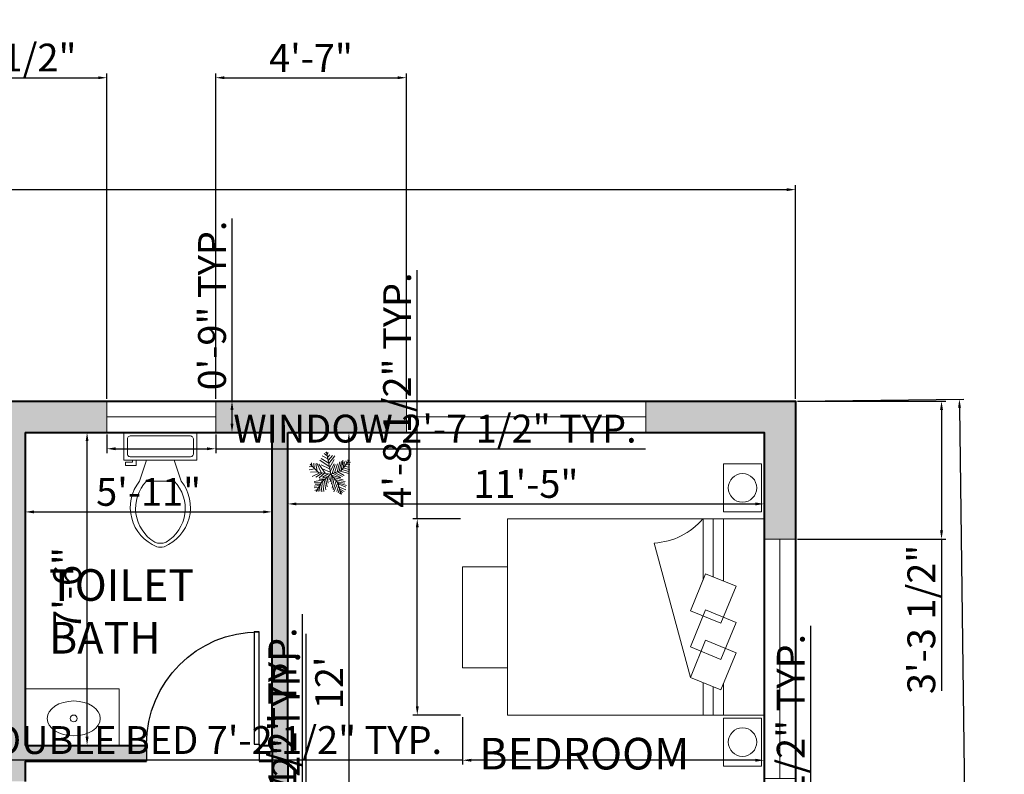
# Model space of a CAD drawing. Units: inches. Extents: x 529 to 1442, y 1029 to 1677.
# Tile 7 of 7: x 1135 to 1418, y 1460 to 1677. Entities that reach past the tile are written whole.
import ezdxf

# ---------------------------------------------------------------- set-up
doc = ezdxf.new("R2010")
doc.units = ezdxf.units.IN
for name, color, linetype, lineweight in [('A-ANNO-DIMS', 2, 'Continuous', 18), ('A-AREA-IDEN', 7, 'Continuous', 25), ('A-DOOR', 4, 'Continuous', 25), ('A-FLOR-FIXT', 9, 'Continuous', 18), ('A-FURN', 8, 'Continuous', 18), ('A-WALL-PATT', 252, 'Continuous', 13), ('tree', 70, 'Continuous', 13), ('wall', 7, 'Continuous', 40), ('window', 52, 'Continuous', 18)]:
    doc.layers.add(name, color=color, linetype=linetype, lineweight=lineweight)
doc.styles.get("Standard").update_dxf_attribs({"font": 'arial.ttf'})
doc.dimstyles.new('ISO-25', dxfattribs={"dimtxt": 8, "dimasz": 2.5, "dimexe": 1.25, "dimexo": 0.625, "dimtad": 1, "dimdec": 0, "dimlunit": 4, "dimtxsty": 'Standard', "dimcen": 2.5, "dimadec": 0, "dimazin": 0, "dimtfac": 1, "dimtdec": 0, "dimtmove": 0, "dimatfit": 3, "dimfxl": 1, "dimarcsym": 0})

# ---------------------------------------------------------------- blocks, each defined once
blk = doc.blocks.new('*U2')
for p, q in [((0, 0), (0, -6)), ((40, 0), (40, -6))]:
    blk.add_line(p, q)
blk.add_lwpolyline([(0, 0), (0, 40), (1.75, 40), (1.75, 0)], close=True)
blk.add_arc((0, 0), 40, 0, 90)
blk = doc.blocks.new('*U4')
for p, q in [((9.5, -6), (9.5, -2)), ((-8, -8.5), (-8, -8)), ((-7, -8), (-7, -9.5)), ((-4, -8), (-6, -14)), ((4, -8), (6, -14)), ((-10, -8.5), (-8, -8.5)), ((-10, -9.5), (-10, -8.5)), ((-7, -9.5), (-10, -9.5)), ((4, -14), (-4, -14))]:
    blk.add_line(p, q)
blk.add_lwpolyline([(10.5, -8), (10.5, 0), (-10.5, 0), (-10.5, -8)], close=True)
for points in [[(-9.5, -2), (-9.5, -6)], [(8.5, -1), (-8.5, -1)], [(-8.5, -7), (8.5, -7)]]:
    blk.add_lwpolyline(points)
for centre, radius, start, end in [((-8.62, -1.88), 0.884, 81.8699, 188.1301), ((8.62, -1.88), 0.884, 351.8699, 98.1301), ((-8.62, -6.12), 0.884, 171.8699, 278.1301), ((8.62, -6.12), 0.884, 261.8699, 8.1301), ((3.52, -21.58), 12.17, 141.4691, 247.9714), ((4.2, -21.82), 11.33, 136.3677, 238.9468), ((-3.52, -21.58), 12.17, 292.0284, 38.5307), ((-4.2, -21.82), 11.33, 301.053, 43.6321), ((0, -27.88), 4, 245.7318, 294.2682), ((0, -29), 4, 254.8605, 285.1395)]:
    blk.add_arc(centre, radius, start, end)
blk = doc.blocks.new('*U12')
for p, q in [((-8.737, 47.138), (-17.069, 52.711)), ((-10.186, 53.64), (-13.084, 55.962)), ((0, 0), (-10.5, 57)), ((-9.099, 51.782), (-6.563, 55.962)), ((-31.5, 4.5), (-52.5, 25.5)), ((-48.585, 21.131), (-49.309, 29.026)), ((-43.513, 28.561), (-42.427, 15.558)), ((-38.442, 26.239), (-34.819, 7.663)), ((-35.544, 28.097), (-24.314, 3.947)), ((-3.665, 19.273), (-27.574, 35.527)), ((-5.114, 28.097), (-24.676, 40.636)), ((-7.288, 39.707), (-21.778, 46.673)), ((-7.65, 43.423), (-2.578, 49.46)), ((-5.839, 35.992), (4.667, 48.067)), ((-5.114, 27.632), (10.463, 46.673)), ((-2.941, 16.486), (8.652, 37.85)), ((-1.129, 6.734), (9.014, 26.704)), ((10.101, 3.483), (17.708, 26.239)), ((16.259, 5.805), (23.142, 31.348)), ((22.055, 7.198), (27.489, 32.277)), ((27, 9), (48, 36)), ((27.127, 9.056), (31.112, 35.992)), ((31.836, 30.883), (32.561, 16.486)), ((35.096, 32.741), (37.27, 22.524)), ((38.719, 34.134), (41.979, 28.561)), ((40.53, 25.775), (48.862, 24.846)), ((43.791, 29.954), (51.036, 30.883)), ((44.153, 36.456), (45.239, 32.741)), ((-47.498, 19.737), (-55.83, 18.344)), ((-40.615, 13.7), (-55.105, 10.913)), ((-33.37, 6.269), (-52.207, 5.34)), ((-28.299, 3.483), (-47.86, -5.805)), ((-21.416, 3.018), (-38.079, -8.128)), ((0, 0), (-31.5, 4.5)), ((-14.533, 2.09), (-30.834, 25.31)), ((-15.982, 2.09), (-30.11, -9.521)), ((-24.314, 23.917), (-2.941, 13.7)), ((0, 0), (-22.5, -19.5)), ((-6.563, 1.161), (-21.416, -8.128)), ((-20.691, 13.7), (-1.129, 4.876)), ((0, 0), (27, 9)), ((0, 0), (18, -22.5)), ((3.942, 1.625), (11.187, 24.381)), ((6.478, 1.625), (26.04, -8.592)), ((11.187, 3.483), (30.749, -5.805)), ((18.07, 5.805), (35.096, -3.483)), ((24.229, 7.663), (46.688, 1.625)), ((29.662, 12.307), (48.137, 6.269)), ((33.285, 16.486), (48.862, 10.913)), ((36.183, 19.737), (48.137, 17.88)), ((-17.431, -15.094), (-42.789, -18.809)), ((-24.314, -21.596), (-42.427, -22.06)), ((-22.5, -19.5), (-37.5, -45)), ((-15.257, -12.772), (-30.11, -12.772)), ((-25.038, -23.918), (-22.865, -45.281)), ((-20.691, -18.345), (-17.793, -44.352)), ((-6.563, -5.805), (-19.967, -9.985)), ((-17.069, -15.094), (-12.721, -40.172)), ((-13.446, -11.378), (-8.737, -32.741)), ((-9.461, -8.592), (-6.201, -23.453)), ((-4.752, -3.483), (-3.665, -14.629)), ((2.493, -3.019), (-1.491, -20.202)), ((1.769, -2.555), (24.229, -9.521)), ((5.029, -6.27), (2.131, -25.775)), ((9.014, -11.378), (3.58, -35.992)), ((14.085, -16.951), (6.478, -40.172)), ((7.565, -9.056), (32.198, -14.629)), ((18.07, -22.524), (8.289, -45.745)), ((12.274, -15.094), (36.907, -18.809)), ((16.259, -19.738), (36.183, -22.989)), ((18, -22.5), (27, -52.5)), ((18.433, -22.524), (40.53, -29.026)), ((19.157, -25.311), (38.719, -33.206)), ((-28.299, -29.026), (-42.789, -31.348)), ((-30.834, -34.135), (-42.427, -35.528)), ((-34.457, -39.708), (-40.978, -42.494)), ((-26.849, -26.24), (-40.253, -25.775)), ((-32.646, -36.921), (-31.921, -44.352)), ((-29.023, -30.884), (-27.936, -43.887)), ((20.244, -30.419), (15.897, -44.816)), ((22.78, -37.85), (19.519, -48.532)), ((21.331, -32.741), (39.081, -40.636)), ((22.78, -38.314), (34.372, -44.816)), ((24.591, -45.745), (23.142, -50.854)), ((24.591, -43.423), (30.749, -47.603)), ((26.764, -49.925), (28.213, -50.854))]:
    blk.add_line(p, q)
blk = doc.blocks.new('*D21')
at = {"layer": 'A-ANNO-DIMS', "color": 0, "lineweight": -2, "transparency": 16777216}
for p, q in [((1136.88, 1557.19), (1136.88, 1533.72)), ((1207.88, 1557.19), (1207.88, 1533.72)), ((1139.38, 1534.97), (1205.38, 1534.97))]:
    blk.add_line(p, q, dxfattribs=at)
at = {"layer": 'A-ANNO-DIMS', "color": 0, "lineweight": 100, "transparency": 16777216}
for points in [[(1139.38, 1535.38), (1139.38, 1534.55), (1136.88, 1534.97)], [(1205.38, 1535.38), (1205.38, 1534.55), (1207.88, 1534.97)]]:
    blk.add_solid(points, dxfattribs=at)
at = {"layer": 'Defpoints', "color": 0, "lineweight": 100, "transparency": 16777216}
for p in [(1136.88, 1557.81), (1207.88, 1557.81), (1207.88, 1534.97)]:
    blk.add_point(p, dxfattribs=at)
at = {"layer": 'A-ANNO-DIMS', "color": 0, "transparency": 16777216, "insert": (1172.38, 1539.68), "char_height": 8, "attachment_point": 5}
blk.add_mtext('5\'-11"', dxfattribs=at)
blk = doc.blocks.new('*D22')
at = {"layer": 'A-ANNO-DIMS', "color": 0, "lineweight": -2, "transparency": 16777216}
for p, q in [((1137.51, 1557.81), (1155.94, 1557.81)), ((1154.69, 1470.31), (1154.69, 1555.31)), ((1137.51, 1467.81), (1155.94, 1467.81))]:
    blk.add_line(p, q, dxfattribs=at)
at = {"layer": 'A-ANNO-DIMS', "color": 0, "lineweight": 100, "transparency": 16777216}
for points in [[(1154.27, 1555.31), (1155.1, 1555.31), (1154.69, 1557.81)], [(1154.27, 1470.31), (1155.1, 1470.31), (1154.69, 1467.81)]]:
    blk.add_solid(points, dxfattribs=at)
at = {"layer": 'Defpoints', "color": 0, "lineweight": 100, "transparency": 16777216}
for p in [(1136.88, 1557.81), (1154.69, 1557.81), (1136.88, 1467.81)]:
    blk.add_point(p, dxfattribs=at)
at = {"layer": 'A-ANNO-DIMS', "color": 0, "transparency": 16777216, "insert": (1149.98, 1512.81), "char_height": 8, "attachment_point": 5, "rotation": 90}
blk.add_mtext('7\'-6"', dxfattribs=at)
blk = doc.blocks.new('*D23')
at = {"layer": 'A-ANNO-DIMS', "color": 0, "lineweight": -2, "transparency": 16777216}
for p, q in [((1212.38, 1557.19), (1212.38, 1536.01)), ((1349.38, 1557.19), (1349.38, 1536.01)), ((1214.88, 1537.26), (1346.88, 1537.26))]:
    blk.add_line(p, q, dxfattribs=at)
at = {"layer": 'A-ANNO-DIMS', "color": 0, "lineweight": 100, "transparency": 16777216}
for points in [[(1214.88, 1537.68), (1214.88, 1536.85), (1212.38, 1537.26)], [(1346.88, 1537.68), (1346.88, 1536.85), (1349.38, 1537.26)]]:
    blk.add_solid(points, dxfattribs=at)
at = {"layer": 'Defpoints', "color": 0, "lineweight": 100, "transparency": 16777216}
for p in [(1212.38, 1557.81), (1349.38, 1557.81), (1349.38, 1537.26)]:
    blk.add_point(p, dxfattribs=at)
at = {"layer": 'A-ANNO-DIMS', "color": 0, "transparency": 16777216, "insert": (1280.88, 1541.97), "char_height": 8, "attachment_point": 5}
blk.add_mtext('11\'-5"', dxfattribs=at)
blk = doc.blocks.new('*D24')
at = {"layer": 'A-ANNO-DIMS', "color": 0, "lineweight": -2, "transparency": 16777216}
for p, q in [((1348.76, 1557.81), (1228.73, 1557.81)), ((1229.98, 1555.31), (1229.98, 1416.31)), ((1348.76, 1413.81), (1228.73, 1413.81))]:
    blk.add_line(p, q, dxfattribs=at)
at = {"layer": 'A-ANNO-DIMS', "color": 0, "lineweight": 100, "transparency": 16777216}
for points in [[(1229.56, 1555.31), (1230.39, 1555.31), (1229.98, 1557.81)], [(1229.56, 1416.31), (1230.39, 1416.31), (1229.98, 1413.81)]]:
    blk.add_solid(points, dxfattribs=at)
at = {"layer": 'Defpoints', "color": 0, "lineweight": 100, "transparency": 16777216}
for p in [(1349.38, 1557.81), (1229.98, 1413.81), (1349.38, 1413.81)]:
    blk.add_point(p, dxfattribs=at)
at = {"layer": 'A-ANNO-DIMS', "color": 0, "transparency": 16777216, "insert": (1225.34, 1485.81), "char_height": 8, "attachment_point": 5, "rotation": 90}
blk.add_mtext("12'", dxfattribs=at)
blk = doc.blocks.new('*D55')
at = {"layer": 'A-ANNO-DIMS', "color": 0, "lineweight": -2, "transparency": 16777216}
for p, q in [((638.38, 1567.44), (638.38, 1628.88)), ((1358.38, 1567.44), (1358.38, 1628.88)), ((640.88, 1627.63), (1355.88, 1627.63))]:
    blk.add_line(p, q, dxfattribs=at)
at = {"layer": 'A-ANNO-DIMS', "color": 0, "lineweight": 100, "transparency": 16777216}
for points in [[(640.88, 1628.05), (640.88, 1627.22), (638.38, 1627.63)], [(1355.88, 1628.05), (1355.88, 1627.22), (1358.38, 1627.63)]]:
    blk.add_solid(points, dxfattribs=at)
at = {"layer": 'Defpoints', "color": 0, "lineweight": 100, "transparency": 16777216}
for p in [(1358.38, 1627.63), (638.38, 1566.81), (1358.38, 1566.81)]:
    blk.add_point(p, dxfattribs=at)
at = {"layer": 'A-ANNO-DIMS', "color": 0, "transparency": 16777216, "insert": (998.38, 1632.34), "char_height": 8, "attachment_point": 5}
blk.add_mtext("60'", dxfattribs=at)
blk = doc.blocks.new('*D56')
at = {"layer": 'A-ANNO-DIMS', "color": 0, "lineweight": -2, "transparency": 16777216}
for p, q in [((1359.01, 1566.82), (1406.77, 1567.43)), ((1405.56, 1564.91), (1410.83, 1149.91)), ((1364.34, 1146.82), (1412.11, 1147.43))]:
    blk.add_line(p, q, dxfattribs=at)
at = {"layer": 'A-ANNO-DIMS', "color": 0, "lineweight": 100, "transparency": 16777216}
for points in [[(1405.97, 1564.92), (1405.14, 1564.91), (1405.52, 1567.41)], [(1411.24, 1149.92), (1410.41, 1149.91), (1410.86, 1147.41)]]:
    blk.add_solid(points, dxfattribs=at)
at = {"layer": 'Defpoints', "color": 0, "lineweight": 100, "transparency": 16777216}
for p in [(1358.38, 1566.81), (1363.72, 1146.81), (1410.86, 1147.41)]:
    blk.add_point(p, dxfattribs=at)
at = {"layer": 'A-ANNO-DIMS', "color": 0, "transparency": 16777216, "insert": (1412.9, 1357.47), "char_height": 8, "attachment_point": 5, "rotation": 270.7276}
blk.add_mtext("35'", dxfattribs=at)
blk = doc.blocks.new('WIN-LARGE-PLAN')
blk.add_line((0, 4.5), (68.85, 4.5))
blk.add_lwpolyline([(0, 9), (68.85, 9), (68.85, 0), (0, 0)], close=True)
blk = doc.blocks.new('WIN-SMALL-PLAN')
blk.add_line((0, 4.5), (31.29, 4.5))
blk.add_lwpolyline([(0, 9), (31.29, 9), (31.29, 0), (0, 0)], close=True)
blk = doc.blocks.new('BED-DOUBLE')
for p, q in [((10.82, 21.21), (49.46, 31.61)), ((0, 17.58), (9.33, 17.58)), ((0, 17.58), (9.33, 17.58)), ((28.37, 17.58), (28.47, 17.58)), ((28.37, 17.58), (28.47, 17.58)), ((38.76, 17.58), (56.44, 17.58)), ((38.76, 17.58), (56.44, 17.58)), ((0, 14.65), (8.12, 14.65)), ((39.74, 14.65), (56.44, 14.65)), ((0, 11.71), (9.09, 11.71)), ((28.13, 11.71), (28.23, 11.71)), ((38.53, 11.71), (56.44, 11.71))]:
    blk.add_line(p, q)
for points in [[(13.54, 73.79), (42.58, 73.79), (42.58, 86.74), (13.54, 86.74)], [(0, 0), (56.44, 0), (56.44, 73.79), (0, 73.79)], [(10.82, 21.21), (21.49, 16.82), (17.9, 8.09), (7.23, 12.48)], [(19.56, 21.21), (30.23, 16.82), (26.64, 8.09), (15.97, 12.48)], [(29.96, 21.21), (40.63, 16.82), (37.04, 8.09), (26.37, 12.48)]]:
    blk.add_lwpolyline(points, close=True)
blk.add_arc((69.23, 32.7), 19.8, 183.1428, 229.758)
blk = doc.blocks.new('NIGHTSTAND')
blk.add_lwpolyline([(0, 0), (13.77, 0), (13.77, 10.99), (0, 10.99)], close=True)
blk.add_circle((6.88, 5.5), 4.1)
blk = doc.blocks.new('WASHBASIN')
blk.add_lwpolyline([(0, 16.29), (27.02, 16.29), (27.02, 0), (0, 0)], close=True)
blk.add_circle((13.05, 8.54), 0.991)
blk.add_ellipse((13.05, 8.54), major_axis=(7.63, 0), ratio=0.659433)
blk = doc.blocks.new('*D73')
at = {"layer": 'A-ANNO-DIMS', "color": 0, "lineweight": -2, "transparency": 16777216}
for p, q in [((1160.38, 1557.19), (1160.38, 1551.87)), ((1191.67, 1557.19), (1191.67, 1551.87)), ((1162.88, 1553.12), (1189.17, 1553.12)), ((1191.67, 1553.12), (1315.29, 1553.12))]:
    blk.add_line(p, q, dxfattribs=at)
at = {"layer": 'A-ANNO-DIMS', "color": 0, "lineweight": 100, "transparency": 16777216}
for points in [[(1162.88, 1553.54), (1162.88, 1552.7), (1160.38, 1553.12)], [(1189.17, 1553.54), (1189.17, 1552.7), (1191.67, 1553.12)]]:
    blk.add_solid(points, dxfattribs=at)
at = {"layer": 'Defpoints', "color": 0, "lineweight": 100, "transparency": 16777216}
for p in [(1160.38, 1557.81), (1191.67, 1557.81), (1191.67, 1553.12)]:
    blk.add_point(p, dxfattribs=at)
at = {"layer": 'A-ANNO-DIMS', "color": 0, "transparency": 16777216, "insert": (1254.73, 1557.88), "char_height": 8, "attachment_point": 5}
blk.add_mtext('WINDOW 2\'-7 1/2" TYP.', dxfattribs=at)
blk = doc.blocks.new('*D74')
at = {"layer": 'A-ANNO-DIMS', "color": 0, "lineweight": -2, "transparency": 16777216}
for p, q in [((1196.36, 1566.81), (1196.36, 1619.33)), ((1192.29, 1566.81), (1197.61, 1566.81)), ((1196.36, 1560.31), (1196.36, 1564.31)), ((1192.29, 1557.81), (1197.61, 1557.81))]:
    blk.add_line(p, q, dxfattribs=at)
at = {"layer": 'A-ANNO-DIMS', "color": 0, "lineweight": 100, "transparency": 16777216}
for points in [[(1195.94, 1564.31), (1196.78, 1564.31), (1196.36, 1566.81)], [(1195.94, 1560.31), (1196.78, 1560.31), (1196.36, 1557.81)]]:
    blk.add_solid(points, dxfattribs=at)
at = {"layer": 'Defpoints', "color": 0, "lineweight": 100, "transparency": 16777216}
for p in [(1191.67, 1566.81), (1196.36, 1566.81), (1191.67, 1557.81)]:
    blk.add_point(p, dxfattribs=at)
at = {"layer": 'A-ANNO-DIMS', "color": 0, "transparency": 16777216, "insert": (1191.65, 1594.32), "char_height": 8, "attachment_point": 5, "rotation": 90}
blk.add_mtext('0\'-9" TYP.', dxfattribs=at)
blk = doc.blocks.new('*D75')
at = {"layer": 'A-ANNO-DIMS', "color": 0, "lineweight": -2, "transparency": 16777216}
for p, q in [((1362.81, 1397.77), (1362.81, 1502.25)), ((1359.01, 1397.77), (1364.06, 1397.77)), ((1362.81, 1370.77), (1362.81, 1395.27)), ((1359.01, 1368.27), (1364.06, 1368.27))]:
    blk.add_line(p, q, dxfattribs=at)
at = {"layer": 'A-ANNO-DIMS', "color": 0, "lineweight": 100, "transparency": 16777216}
for points in [[(1362.39, 1395.27), (1363.23, 1395.27), (1362.81, 1397.77)], [(1362.39, 1370.77), (1363.23, 1370.77), (1362.81, 1368.27)]]:
    blk.add_solid(points, dxfattribs=at)
at = {"layer": 'Defpoints', "color": 0, "lineweight": 100, "transparency": 16777216}
for p in [(1358.38, 1397.77), (1362.81, 1397.77), (1358.38, 1368.27)]:
    blk.add_point(p, dxfattribs=at)
at = {"layer": 'A-ANNO-DIMS', "color": 0, "transparency": 16777216, "insert": (1358.05, 1451.26), "char_height": 8, "attachment_point": 5, "rotation": 90}
blk.add_mtext('VENT 2\'-5 1/2" TYP.', dxfattribs=at)
blk = doc.blocks.new('*D77')
at = {"layer": 'A-ANNO-DIMS', "color": 0, "lineweight": -2, "transparency": 16777216}
for p, q in [((1262.64, 1475.94), (1262.64, 1462.3)), ((1349.38, 1475.94), (1349.38, 1462.3)), ((1262.64, 1463.55), (1116.74, 1463.55)), ((1346.88, 1463.55), (1265.14, 1463.55))]:
    blk.add_line(p, q, dxfattribs=at)
at = {"layer": 'A-ANNO-DIMS', "color": 0, "lineweight": 100, "transparency": 16777216}
for points in [[(1265.14, 1463.97), (1265.14, 1463.13), (1262.64, 1463.55)], [(1346.88, 1463.97), (1346.88, 1463.13), (1349.38, 1463.55)]]:
    blk.add_solid(points, dxfattribs=at)
at = {"layer": 'Defpoints', "color": 0, "lineweight": 100, "transparency": 16777216}
for p in [(1262.64, 1476.56), (1349.38, 1476.56), (1262.64, 1463.55)]:
    blk.add_point(p, dxfattribs=at)
at = {"layer": 'A-ANNO-DIMS', "color": 0, "transparency": 16777216, "insert": (1188.44, 1468.32), "char_height": 8, "attachment_point": 5}
blk.add_mtext('DOUBLE BED 7\'-2 1/2" TYP.', dxfattribs=at)
blk = doc.blocks.new('*D78')
at = {"layer": 'A-ANNO-DIMS', "color": 0, "lineweight": -2, "transparency": 16777216}
for p, q in [((1249.63, 1533), (1249.63, 1604.48)), ((1262.02, 1533), (1248.38, 1533)), ((1249.63, 1479.06), (1249.63, 1530.5)), ((1262.02, 1476.56), (1248.38, 1476.56))]:
    blk.add_line(p, q, dxfattribs=at)
at = {"layer": 'A-ANNO-DIMS', "color": 0, "lineweight": 100, "transparency": 16777216}
for points in [[(1249.22, 1530.5), (1250.05, 1530.5), (1249.63, 1533)], [(1249.22, 1479.06), (1250.05, 1479.06), (1249.63, 1476.56)]]:
    blk.add_solid(points, dxfattribs=at)
at = {"layer": 'Defpoints', "color": 0, "lineweight": 100, "transparency": 16777216}
for p in [(1249.63, 1533), (1262.64, 1533), (1262.64, 1476.56)]:
    blk.add_point(p, dxfattribs=at)
at = {"layer": 'A-ANNO-DIMS', "color": 0, "transparency": 16777216, "insert": (1244.87, 1569.99), "char_height": 8, "attachment_point": 5, "rotation": 90}
blk.add_mtext('4\'-8 1/2" TYP.', dxfattribs=at)
blk = doc.blocks.new('*D87')
at = {"layer": 'A-ANNO-DIMS', "color": 0, "lineweight": -2, "transparency": 16777216}
for p, q in [((1216.62, 1371.24), (1216.62, 1505.58)), ((1213.45, 1371.24), (1217.87, 1371.24)), ((1216.62, 1348.45), (1216.62, 1368.74)), ((1213.45, 1345.95), (1217.87, 1345.95))]:
    blk.add_line(p, q, dxfattribs=at)
at = {"layer": 'A-ANNO-DIMS', "color": 0, "lineweight": 100, "transparency": 16777216}
for points in [[(1216.2, 1368.74), (1217.04, 1368.74), (1216.62, 1371.24)], [(1216.2, 1348.45), (1217.04, 1348.45), (1216.62, 1345.95)]]:
    blk.add_solid(points, dxfattribs=at)
at = {"layer": 'Defpoints', "color": 0, "lineweight": 100, "transparency": 16777216}
for p in [(1212.83, 1371.24), (1216.62, 1371.24), (1212.83, 1345.95)]:
    blk.add_point(p, dxfattribs=at)
at = {"layer": 'A-ANNO-DIMS', "color": 0, "transparency": 16777216, "insert": (1211.86, 1439.66), "char_height": 8, "attachment_point": 5, "rotation": 90}
blk.add_mtext('ARMCHAIR 2\'-1 1/2" TYP.', dxfattribs=at)
blk = doc.blocks.new('*D91')
at = {"layer": 'A-ANNO-DIMS', "color": 0, "lineweight": -2, "transparency": 16777216}
for p, q in [((1217.67, 1335.7), (1217.67, 1499.91)), ((1212.96, 1335.7), (1218.92, 1335.7)), ((1217.67, 1302.63), (1217.67, 1333.2)), ((1212.96, 1300.13), (1218.92, 1300.13))]:
    blk.add_line(p, q, dxfattribs=at)
at = {"layer": 'A-ANNO-DIMS', "color": 0, "lineweight": 100, "transparency": 16777216}
for points in [[(1217.25, 1333.2), (1218.08, 1333.2), (1217.67, 1335.7)], [(1217.25, 1302.63), (1218.08, 1302.63), (1217.67, 1300.13)]]:
    blk.add_solid(points, dxfattribs=at)
at = {"layer": 'Defpoints', "color": 0, "lineweight": 100, "transparency": 16777216}
for p in [(1212.33, 1335.7), (1217.67, 1335.7), (1212.33, 1300.13)]:
    blk.add_point(p, dxfattribs=at)
at = {"layer": 'A-ANNO-DIMS', "color": 0, "transparency": 16777216, "insert": (1212.9, 1419.05), "char_height": 8, "attachment_point": 5, "rotation": 90}
blk.add_mtext('COFFEE TABLE 2\'-11 1/2" TYP.', dxfattribs=at)
blk = doc.blocks.new('*D103')
at = {"layer": 'A-ANNO-DIMS', "color": 0, "lineweight": -2, "transparency": 16777216}
for p, q in [((1099.95, 1567.44), (1099.95, 1661.06)), ((1102.45, 1659.81), (1157.88, 1659.81)), ((1160.38, 1567.44), (1160.38, 1661.06))]:
    blk.add_line(p, q, dxfattribs=at)
at = {"layer": 'A-ANNO-DIMS', "color": 0, "lineweight": 100, "transparency": 16777216}
for points in [[(1102.45, 1660.23), (1102.45, 1659.4), (1099.95, 1659.81)], [(1157.88, 1660.23), (1157.88, 1659.4), (1160.38, 1659.81)]]:
    blk.add_solid(points, dxfattribs=at)
at = {"layer": 'Defpoints', "color": 0, "lineweight": 100, "transparency": 16777216}
for p in [(1160.38, 1659.81), (1099.95, 1566.81), (1160.38, 1566.81)]:
    blk.add_point(p, dxfattribs=at)
at = {"layer": 'A-ANNO-DIMS', "color": 0, "transparency": 16777216, "insert": (1130.17, 1664.57), "char_height": 8, "attachment_point": 5}
blk.add_mtext('5\'-0 1/2"', dxfattribs=at)
blk = doc.blocks.new('*D104')
at = {"layer": 'A-ANNO-DIMS', "color": 0, "lineweight": -2, "transparency": 16777216}
for p, q in [((1191.67, 1567.44), (1191.67, 1661.06)), ((1194.17, 1659.81), (1244, 1659.81)), ((1246.5, 1567.44), (1246.5, 1661.06))]:
    blk.add_line(p, q, dxfattribs=at)
at = {"layer": 'A-ANNO-DIMS', "color": 0, "lineweight": 100, "transparency": 16777216}
for points in [[(1194.17, 1660.23), (1194.17, 1659.4), (1191.67, 1659.81)], [(1244, 1660.23), (1244, 1659.4), (1246.5, 1659.81)]]:
    blk.add_solid(points, dxfattribs=at)
at = {"layer": 'Defpoints', "color": 0, "lineweight": 100, "transparency": 16777216}
for p in [(1246.5, 1659.81), (1191.67, 1566.81), (1246.5, 1566.81)]:
    blk.add_point(p, dxfattribs=at)
at = {"layer": 'A-ANNO-DIMS', "color": 0, "transparency": 16777216, "insert": (1219.08, 1664.44), "char_height": 8, "attachment_point": 5}
blk.add_mtext('4\'-7"', dxfattribs=at)
blk = doc.blocks.new('*D108')
at = {"layer": 'A-ANNO-DIMS', "color": 0, "lineweight": -2, "transparency": 16777216}
for p, q in [((1359.01, 1566.81), (1401.63, 1566.81)), ((1400.38, 1564.31), (1400.38, 1529.64)), ((1359.01, 1527.14), (1401.63, 1527.14)), ((1400.38, 1527.14), (1400.38, 1483.49))]:
    blk.add_line(p, q, dxfattribs=at)
at = {"layer": 'A-ANNO-DIMS', "color": 0, "lineweight": 100, "transparency": 16777216}
for points in [[(1399.97, 1564.31), (1400.8, 1564.31), (1400.38, 1566.81)], [(1399.97, 1529.64), (1400.8, 1529.64), (1400.38, 1527.14)]]:
    blk.add_solid(points, dxfattribs=at)
at = {"layer": 'Defpoints', "color": 0, "lineweight": 100, "transparency": 16777216}
for p in [(1358.38, 1566.81), (1358.38, 1527.14), (1400.38, 1527.14)]:
    blk.add_point(p, dxfattribs=at)
at = {"layer": 'A-ANNO-DIMS', "color": 0, "transparency": 16777216, "insert": (1395.62, 1504.06), "char_height": 8, "attachment_point": 5, "rotation": 90}
blk.add_mtext('3\'-3 1/2"', dxfattribs=at)

msp = doc.modelspace()

# ---------------------------------------------------------------- hatches: boundary and pattern name
at = {"layer": 'A-WALL-PATT'}
h = msp.add_hatch(color=256, dxfattribs=at)
h.dxf.hatch_style = 1
h.paths.add_polyline_path([(1132.38, 1328.31), (1041.38, 1328.31), (1041.38, 1323.81), (1132.38, 1323.81)])
h.paths.add_polyline_path([(1132.38, 1413.81), (1075.12, 1413.81), (1075.12, 1409.31), (1132.38, 1409.31)])
h.paths.add_polyline_path([(1246.5, 1566.81), (1191.67, 1566.81), (1191.67, 1557.81), (1246.5, 1557.81)])
h.paths.add_polyline_path([(1160.38, 1566.81), (1099.95, 1566.81), (1099.95, 1557.81), (1132.38, 1557.81), (1160.38, 1557.81)])
h = msp.add_hatch(color=256, dxfattribs=at)
h.dxf.hatch_style = 1
h.paths.add_polyline_path([(1160.38, 1566.81), (1099.95, 1566.81), (1099.95, 1557.81), (1132.38, 1557.81), (1160.38, 1557.81)])
h.paths.add_polyline_path([(1136.88, 1557.81), (1132.38, 1557.81), (1132.38, 1457.46), (1136.88, 1457.46)])
h.paths.add_polyline_path([(1171.8, 1467.81), (1136.88, 1467.81), (1136.88, 1463.31), (1171.8, 1463.31)])
h.paths.add_polyline_path([(1212.38, 1557.81), (1207.88, 1557.81), (1207.88, 1467.81), (1207.88, 1409.31), (1218.04, 1409.31), (1218.04, 1413.81), (1212.38, 1413.81), (1212.38, 1463.31)])
h.paths.add_polyline_path([(1136.88, 1409.31), (1132.38, 1409.31), (1132.38, 1146.81), (1136.88, 1146.81)])
h.paths.add_polyline_path([(1136.88, 1417.46), (1132.38, 1417.46), (1132.38, 1409.31), (1136.88, 1409.31)])
h.paths.add_polyline_path([(1132.38, 1413.81), (1075.12, 1413.81), (1075.12, 1409.31), (1132.38, 1409.31)])
h.paths.add_polyline_path([(1132.38, 1328.31), (1041.38, 1328.31), (1041.38, 1323.81), (1132.38, 1323.81)])
h = msp.add_hatch(color=256, dxfattribs=at)
h.dxf.hatch_style = 1
h.paths.add_polyline_path([(1358.38, 1566.81), (1315.35, 1566.81), (1315.35, 1557.81), (1349.38, 1557.81), (1349.38, 1527.14), (1358.38, 1527.14)])
h = msp.add_hatch(color=256, dxfattribs=at)
h.dxf.hatch_style = 1
h.paths.add_polyline_path([(1171.8, 1467.81), (1136.88, 1467.81), (1136.88, 1463.31), (1171.8, 1463.31)])
h.paths.add_polyline_path([(1136.88, 1557.81), (1132.38, 1557.81), (1132.38, 1457.46), (1136.88, 1457.46)])
h.paths.add_polyline_path([(1212.38, 1557.81), (1207.88, 1557.81), (1207.88, 1467.81), (1207.88, 1409.31), (1218.04, 1409.31), (1218.04, 1413.81), (1212.38, 1413.81), (1212.38, 1463.31)])

# ---------------------------------------------------------------- linework, layer by layer
at = {"layer": 'wall'}
for p, q in [((638.38, 1566.81), (1358.38, 1566.81)), ((1358.38, 1566.81), (1358.38, 1146.81)), ((1136.88, 1557.81), (1136.88, 1467.81)), ((1136.88, 1557.81), (1136.88, 1467.81)), ((1207.88, 1467.81), (1207.88, 1557.81)), ((1212.38, 1463.31), (1212.38, 1557.81)), ((1349.38, 1557.81), (1349.38, 1413.81)), ((1136.88, 1467.81), (1171.8, 1467.81)), ((1204.13, 1467.81), (1207.88, 1467.81)), ((1207.88, 1467.81), (1207.88, 1409.31)), ((1136.88, 1463.31), (1171.8, 1463.31)), ((1136.88, 1463.31), (1136.88, 1457.46)), ((1204.13, 1463.31), (1207.88, 1463.31)), ((1212.38, 1463.31), (1212.38, 1413.81))]:
    msp.add_line(p, q, dxfattribs=at)
for points in [[(859.38, 1146.81), (638.38, 1146.81), (638.38, 1566.81), (1358.38, 1566.81), (1358.38, 1146.81), (1132.38, 1146.81)], [(1136.88, 1557.81), (1207.88, 1557.81)], [(1212.38, 1557.81), (1349.38, 1557.81), (1349.38, 1253.97)]]:
    msp.add_lwpolyline(points, dxfattribs=at)

# ---------------------------------------------------------------- block references
at = {"layer": 'A-DOOR', "xscale": -0.8082241798979204, "yscale": 0.8082241798979204, "zscale": 0.8082241798979204}
msp.add_blockref('*U2', (1204.13, 1468.16), dxfattribs=at)
at = {"layer": 'A-FLOR-FIXT'}
msp.add_blockref('*U4', (1175.77, 1557.81), dxfattribs=at)
at = {"layer": 'A-FLOR-FIXT', "rotation": 180}
msp.add_blockref('WASHBASIN', (1163.9, 1484.1), dxfattribs=at)
msp.add_blockref('WASHBASIN', (1163.9, 1484.1), dxfattribs=at)
at = {"layer": 'A-FURN'}
for name, p, rotation in [('NIGHTSTAND', (1348.66, 1534.99), 89.99999999999616), ('BED-DOUBLE', (1349.38, 1476.56), 90.0000000000003), ('NIGHTSTAND', (1348.66, 1461.89), 89.99999999999456)]:
    msp.add_blockref(name, p, dxfattribs=dict(at, rotation=rotation))
at = {"layer": 'tree', "xscale": 0.1116431773080361, "yscale": 0.1116431773080361, "zscale": 0.1116431773080361}
msp.add_blockref('*U12', (1224.74, 1545.83), dxfattribs=at)
at = {"layer": 'window'}
for name, p in [('WIN-SMALL-PLAN', (1160.38, 1557.81)), ('WIN-LARGE-PLAN', (1246.5, 1557.81))]:
    msp.add_blockref(name, p, dxfattribs=at)
at = {"layer": 'window', "rotation": 269.9999999999987}
msp.add_blockref('WIN-LARGE-PLAN', (1349.38, 1527.14), dxfattribs=at)

# ---------------------------------------------------------------- texts
at = {"layer": 'A-AREA-IDEN', "char_height": 9.098, "attachment_point": 1}
for s, insert in [('TOILET\\PBATH', (1143.71, 1518.49)), ('BEDROOM', (1267.45, 1469.99))]:
    msp.add_mtext_dynamic_manual_height_columns(s, width=307.5887, gutter_width=45.49, heights=[0], dxfattribs=dict(at, insert=insert))

# ---------------------------------------------------------------- dimensions: what is measured, and where the dimension line sits
at = {"layer": 'A-ANNO-DIMS'}
for base, p1, p2, override, picture, middle in [((1160.38, 1659.81), (1099.95, 1566.81), (1160.38, 1566.81), {"dimdec": 1, "dimlfac": 1, "dimrnd": 0, "dimzin": 1, "dimdsep": 46, "dimlunit": 4, "dimfrac": 2}, '*D103', (1130.17, 1664.57)), ((1246.5, 1659.81), (1191.67, 1566.81), (1246.5, 1566.81), {"dimdec": 1, "dimlfac": 1, "dimrnd": 0, "dimzin": 1, "dimdsep": 46, "dimlunit": 4, "dimfrac": 2}, '*D104', (1219.08, 1664.44)), ((1358.38, 1627.63), (638.38, 1566.81), (1358.38, 1566.81), {"dimclrd": 0, "dimclre": 0, "dimclrt": 0}, '*D55', (998.38, 1632.34)), ((1207.88, 1534.97), (1136.88, 1557.81), (1207.88, 1557.81), {"dimclrd": 0, "dimclre": 0, "dimclrt": 0}, '*D21', (1172.38, 1539.68)), ((1349.38, 1537.26), (1212.38, 1557.81), (1349.38, 1557.81), {"dimclrd": 0, "dimclre": 0, "dimclrt": 0}, '*D23', (1280.88, 1541.97))]:
    dim = msp.add_linear_dim(base=base, p1=p1, p2=p2, dimstyle='ISO-25', override=override, dxfattribs=at)
    dim.commit()
    dim.dimension.update_dxf_attribs({"geometry": picture, "text_midpoint": middle})
for base, p1, p2, angle, text, picture, middle in [((1196.36, 1566.81), (1191.67, 1557.81), (1191.67, 1566.81), 90, '<> TYP.', '*D74', (1191.65, 1594.32)), ((1249.63, 1533), (1262.64, 1476.56), (1262.64, 1533), 90, '<> TYP.', '*D78', (1244.87, 1569.99)), ((1216.62, 1371.24), (1212.83, 1345.95), (1212.83, 1371.24), 90, 'ARMCHAIR <> TYP.', '*D87', (1211.86, 1439.66)), ((1362.81, 1397.77), (1358.38, 1368.27), (1358.38, 1397.77), 90, 'VENT <> TYP.', '*D75', (1358.05, 1451.26)), ((1262.64, 1463.55), (1349.38, 1476.56), (1262.64, 1476.56), 180, 'DOUBLE BED <> TYP.', '*D77', (1188.44, 1468.32)), ((1217.67, 1335.7), (1212.33, 1300.13), (1212.33, 1335.7), 90, 'COFFEE TABLE <> TYP.', '*D91', (1212.9, 1419.05))]:
    dim = msp.add_linear_dim(base=base, p1=p1, p2=p2, angle=angle, text=text, dimstyle='ISO-25', override={"dimdec": 1, "dimlfac": 1, "dimrnd": 0, "dimzin": 1, "dimdsep": 46, "dimlunit": 4, "dimfrac": 2}, dxfattribs=at)
    dim.commit()
    dim.dimension.update_dxf_attribs({"geometry": picture, "text_midpoint": middle})
dim = msp.add_linear_dim(base=(1191.67, 1553.12), p1=(1160.38, 1557.81), p2=(1191.67, 1557.81), text='WINDOW <> TYP.', dimstyle='ISO-25', override={"dimdec": 1, "dimlfac": 1, "dimrnd": 0, "dimzin": 1, "dimdsep": 46, "dimlunit": 4, "dimfrac": 2}, dxfattribs=at)
dim.commit()
dim.dimension.update_dxf_attribs({"geometry": '*D73', "text_midpoint": (1254.73, 1557.88)})
dim = msp.add_aligned_dim(p1=(1358.38, 1566.81), p2=(1363.72, 1146.81), distance=47.14, dimstyle='ISO-25', override={"dimclrd": 0, "dimclre": 0, "dimclrt": 0}, dxfattribs=at)
dim.commit()
dim.dimension.update_dxf_attribs({"geometry": '*D56', "text_midpoint": (1412.9, 1357.47)})
for base, p1, p2, override, picture, middle in [((1400.38, 1527.14), (1358.38, 1566.81), (1358.38, 1527.14), {"dimdec": 1, "dimlfac": 1, "dimrnd": 0, "dimzin": 1, "dimdsep": 46, "dimlunit": 4, "dimfrac": 2}, '*D108', (1395.62, 1504.06)), ((1154.69, 1557.81), (1136.88, 1467.81), (1136.88, 1557.81), {"dimclrd": 0, "dimclre": 0, "dimclrt": 0}, '*D22', (1149.98, 1512.81)), ((1229.98, 1413.81), (1349.38, 1557.81), (1349.38, 1413.81), {"dimclrd": 0, "dimclre": 0, "dimclrt": 0}, '*D24', (1225.34, 1485.81))]:
    dim = msp.add_linear_dim(base=base, p1=p1, p2=p2, angle=90, dimstyle='ISO-25', override=override, dxfattribs=at)
    dim.commit()
    dim.dimension.update_dxf_attribs({"geometry": picture, "text_midpoint": middle})

doc.saveas('drawing.dxf')
